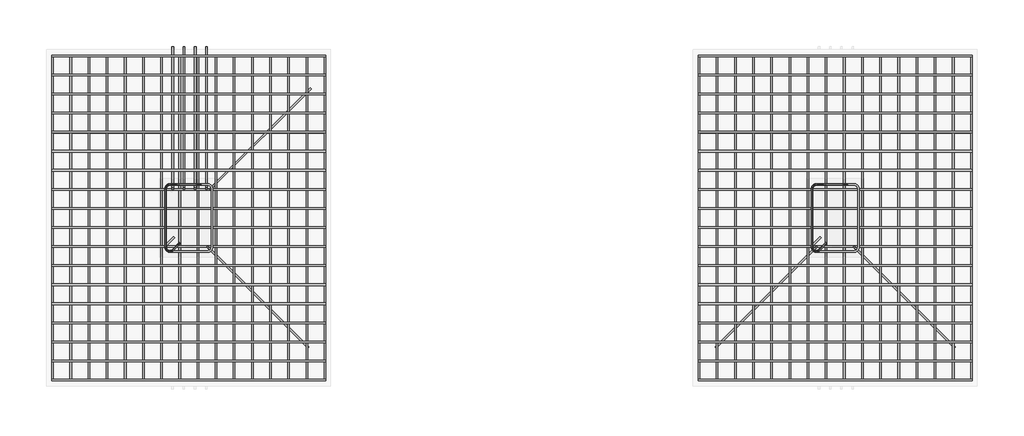
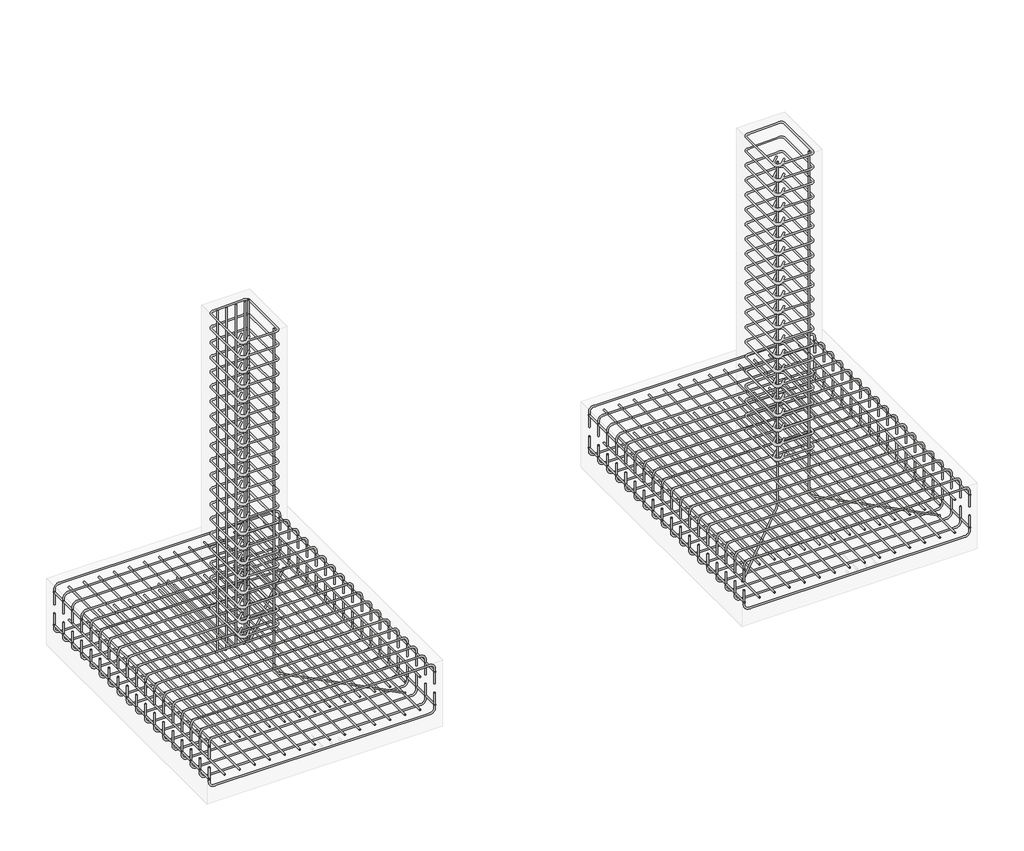
# One storey, part 10 of 33: 15 reinforcing bars.
"""IFC4 building model written with IfcOpenShell, lengths in millimetres."""

from ifc_helpers import new_model, si_unit, point, frame, origin, place, context, project, spatial, polyline, circle_curve, trimmed, segment, composite_curve, source, transform, mapped, element, save
from ifc_brep_helpers import swept_disk

model = new_model("IFC4")

# Units and contexts
model_context = context("Model", 3, world=origin())
ifc_project = project(units=[si_unit("LENGTHUNIT", "METRE", prefix="MILLI")], contexts=[model_context])

# Site, building, storey
site = spatial("IfcSite", under=ifc_project)
building = spatial("IfcBuilding", under=site)
storey = spatial("IfcBuildingStorey", under=building, Elevation=-3000.0)

# Reinforcing bars
placement = place(None, origin())
reinforcing_bar_shape = source(origin(), model_context, "Body", "SolidModel", [
    swept_disk(composite_curve([segment(polyline([(14306.5357258, -2044.0608134, -3240.0), (14306.5357258, -2044.0608134, -3092.7)]), True, "CONTINUOUS"), segment(trimmed(circle_curve(frame((14352.8857258, -2044.0608134, -3092.7), z_axis=(0.0, 1.0, 0.0), x_axis=(-46.350000000000364, 0.0, 0.0)), 46.35), [point((14306.5357258, -2044.0608134, -3092.7))], [point((14352.8857258, -2044.0608134, -3046.35))], True, "CARTESIAN"), True, "CONTINUOUS"), segment(polyline([(14352.8857258, -2044.0608134, -3046.35), (16367.4857258, -2044.0608134, -3046.35)]), True, "CONTINUOUS"), segment(trimmed(circle_curve(frame((16367.4857258, -2044.0608134, -3092.7), z_axis=(0.0, 1.0, 0.0), x_axis=(0.0, 0.0, 46.34999999999991)), 46.35), [point((16367.4857258, -2044.0608134, -3046.35))], [point((16413.8357258, -2044.0608134, -3092.7))], True, "CARTESIAN"), True, "CONTINUOUS"), segment(polyline([(16413.8357258, -2044.0608134, -3092.7), (16413.8357258, -2044.0608134, -3240.0)]), True, "CONTINUOUS")], self_intersect=False), 6.35),
])
element("IfcReinforcingBar", 1, at=placement, inside=storey, context=model_context, shape_type="MappedRepresentation", body=[
    mapped(reinforcing_bar_shape, transform((0.0, 0.0, 0.0), x_axis=(1.0, 0.0, 0.0), y_axis=(0.0, 1.0, 0.0), z_axis=(0.0, 0.0, 1.0))),
    mapped(reinforcing_bar_shape, transform((0.0, -147.4882353, 0.0), x_axis=(1.0, 0.0, 0.0), y_axis=(0.0, 1.0, 0.0), z_axis=(0.0, 0.0, 1.0))),
    mapped(reinforcing_bar_shape, transform((0.0, -294.9764706, 0.0), x_axis=(1.0, 0.0, 0.0), y_axis=(0.0, 1.0, 0.0), z_axis=(0.0, 0.0, 1.0))),
    mapped(reinforcing_bar_shape, transform((0.0, -442.4647059, 0.0), x_axis=(1.0, 0.0, 0.0), y_axis=(0.0, 1.0, 0.0), z_axis=(0.0, 0.0, 1.0))),
    mapped(reinforcing_bar_shape, transform((0.0, -589.9529412, 0.0), x_axis=(1.0, 0.0, 0.0), y_axis=(0.0, 1.0, 0.0), z_axis=(0.0, 0.0, 1.0))),
    mapped(reinforcing_bar_shape, transform((0.0, -737.4411765, 0.0), x_axis=(1.0, 0.0, 0.0), y_axis=(0.0, 1.0, 0.0), z_axis=(0.0, 0.0, 1.0))),
    mapped(reinforcing_bar_shape, transform((0.0, -884.9294118, 0.0), x_axis=(1.0, 0.0, 0.0), y_axis=(0.0, 1.0, 0.0), z_axis=(0.0, 0.0, 1.0))),
    mapped(reinforcing_bar_shape, transform((0.0, -1032.4176471, 0.0), x_axis=(1.0, 0.0, 0.0), y_axis=(0.0, 1.0, 0.0), z_axis=(0.0, 0.0, 1.0))),
    mapped(reinforcing_bar_shape, transform((0.0, -1179.9058824, 0.0), x_axis=(1.0, 0.0, 0.0), y_axis=(0.0, 1.0, 0.0), z_axis=(0.0, 0.0, 1.0))),
    mapped(reinforcing_bar_shape, transform((0.0, -1327.3941176, 0.0), x_axis=(1.0, 0.0, 0.0), y_axis=(0.0, 1.0, 0.0), z_axis=(0.0, 0.0, 1.0))),
    mapped(reinforcing_bar_shape, transform((0.0, -1474.8823529, 0.0), x_axis=(1.0, 0.0, 0.0), y_axis=(0.0, 1.0, 0.0), z_axis=(0.0, 0.0, 1.0))),
    mapped(reinforcing_bar_shape, transform((0.0, -1622.3705882, 0.0), x_axis=(1.0, 0.0, 0.0), y_axis=(0.0, 1.0, 0.0), z_axis=(0.0, 0.0, 1.0))),
    mapped(reinforcing_bar_shape, transform((0.0, -1769.8588235, 0.0), x_axis=(1.0, 0.0, 0.0), y_axis=(0.0, 1.0, 0.0), z_axis=(0.0, 0.0, 1.0))),
    mapped(reinforcing_bar_shape, transform((0.0, -1917.3470588, 0.0), x_axis=(1.0, 0.0, 0.0), y_axis=(0.0, 1.0, 0.0), z_axis=(0.0, 0.0, 1.0))),
    mapped(reinforcing_bar_shape, transform((0.0, -2064.8352941, 0.0), x_axis=(1.0, 0.0, 0.0), y_axis=(0.0, 1.0, 0.0), z_axis=(0.0, 0.0, 1.0))),
    mapped(reinforcing_bar_shape, transform((0.0, -2212.3235294, 0.0), x_axis=(1.0, 0.0, 0.0), y_axis=(0.0, 1.0, 0.0), z_axis=(0.0, 0.0, 1.0))),
    mapped(reinforcing_bar_shape, transform((0.0, -2359.8117647, 0.0), x_axis=(1.0, 0.0, 0.0), y_axis=(0.0, 1.0, 0.0), z_axis=(0.0, 0.0, 1.0))),
    mapped(reinforcing_bar_shape, transform((0.0, -2507.3, 0.0), x_axis=(1.0, 0.0, 0.0), y_axis=(0.0, 1.0, 0.0), z_axis=(0.0, 0.0, 1.0))),
])
reinforcing_bar_2_shape = source(origin(), model_context, "Body", "SolidModel", [
    swept_disk(composite_curve([segment(polyline([(16413.8357258, -2044.0608134, -3330.080452), (16413.8357258, -2044.0608134, -3477.380452)]), True, "CONTINUOUS"), segment(trimmed(circle_curve(frame((16367.4857258, -2044.0608134, -3477.380452), z_axis=(0.0, 1.0, 0.0), x_axis=(46.350000000000364, 0.0, 0.0)), 46.35), [point((16413.8357258, -2044.0608134, -3477.380452))], [point((16367.4857258, -2044.0608134, -3523.730452))], True, "CARTESIAN"), True, "CONTINUOUS"), segment(polyline([(16367.4857258, -2044.0608134, -3523.730452), (14352.8857258, -2044.0608134, -3523.730452)]), True, "CONTINUOUS"), segment(trimmed(circle_curve(frame((14352.8857258, -2044.0608134, -3477.380452), z_axis=(0.0, 1.0, 0.0), x_axis=(0.0, 0.0, -46.34999999999991)), 46.35), [point((14352.8857258, -2044.0608134, -3523.730452))], [point((14306.5357258, -2044.0608134, -3477.380452))], True, "CARTESIAN"), True, "CONTINUOUS"), segment(polyline([(14306.5357258, -2044.0608134, -3477.380452), (14306.5357258, -2044.0608134, -3330.080452)]), True, "CONTINUOUS")], self_intersect=False), 6.35),
])
element("IfcReinforcingBar", 2, at=placement, inside=storey, context=model_context, shape_type="MappedRepresentation", body=[
    mapped(reinforcing_bar_2_shape, transform((0.0, 0.0, 0.0), x_axis=(1.0, 0.0, 0.0), y_axis=(0.0, 1.0, 0.0), z_axis=(0.0, 0.0, 1.0))),
    mapped(reinforcing_bar_2_shape, transform((0.0, -147.4882353, 0.0), x_axis=(1.0, 0.0, 0.0), y_axis=(0.0, 1.0, 0.0), z_axis=(0.0, 0.0, 1.0))),
    mapped(reinforcing_bar_2_shape, transform((0.0, -294.9764706, 0.0), x_axis=(1.0, 0.0, 0.0), y_axis=(0.0, 1.0, 0.0), z_axis=(0.0, 0.0, 1.0))),
    mapped(reinforcing_bar_2_shape, transform((0.0, -442.4647059, 0.0), x_axis=(1.0, 0.0, 0.0), y_axis=(0.0, 1.0, 0.0), z_axis=(0.0, 0.0, 1.0))),
    mapped(reinforcing_bar_2_shape, transform((0.0, -589.9529412, 0.0), x_axis=(1.0, 0.0, 0.0), y_axis=(0.0, 1.0, 0.0), z_axis=(0.0, 0.0, 1.0))),
    mapped(reinforcing_bar_2_shape, transform((0.0, -737.4411765, 0.0), x_axis=(1.0, 0.0, 0.0), y_axis=(0.0, 1.0, 0.0), z_axis=(0.0, 0.0, 1.0))),
    mapped(reinforcing_bar_2_shape, transform((0.0, -884.9294118, 0.0), x_axis=(1.0, 0.0, 0.0), y_axis=(0.0, 1.0, 0.0), z_axis=(0.0, 0.0, 1.0))),
    mapped(reinforcing_bar_2_shape, transform((0.0, -1032.4176471, 0.0), x_axis=(1.0, 0.0, 0.0), y_axis=(0.0, 1.0, 0.0), z_axis=(0.0, 0.0, 1.0))),
    mapped(reinforcing_bar_2_shape, transform((0.0, -1179.9058824, 0.0), x_axis=(1.0, 0.0, 0.0), y_axis=(0.0, 1.0, 0.0), z_axis=(0.0, 0.0, 1.0))),
    mapped(reinforcing_bar_2_shape, transform((0.0, -1327.3941176, 0.0), x_axis=(1.0, 0.0, 0.0), y_axis=(0.0, 1.0, 0.0), z_axis=(0.0, 0.0, 1.0))),
    mapped(reinforcing_bar_2_shape, transform((0.0, -1474.8823529, 0.0), x_axis=(1.0, 0.0, 0.0), y_axis=(0.0, 1.0, 0.0), z_axis=(0.0, 0.0, 1.0))),
    mapped(reinforcing_bar_2_shape, transform((0.0, -1622.3705882, 0.0), x_axis=(1.0, 0.0, 0.0), y_axis=(0.0, 1.0, 0.0), z_axis=(0.0, 0.0, 1.0))),
    mapped(reinforcing_bar_2_shape, transform((0.0, -1769.8588235, 0.0), x_axis=(1.0, 0.0, 0.0), y_axis=(0.0, 1.0, 0.0), z_axis=(0.0, 0.0, 1.0))),
    mapped(reinforcing_bar_2_shape, transform((0.0, -1917.3470588, 0.0), x_axis=(1.0, 0.0, 0.0), y_axis=(0.0, 1.0, 0.0), z_axis=(0.0, 0.0, 1.0))),
    mapped(reinforcing_bar_2_shape, transform((0.0, -2064.8352941, 0.0), x_axis=(1.0, 0.0, 0.0), y_axis=(0.0, 1.0, 0.0), z_axis=(0.0, 0.0, 1.0))),
    mapped(reinforcing_bar_2_shape, transform((0.0, -2212.3235294, 0.0), x_axis=(1.0, 0.0, 0.0), y_axis=(0.0, 1.0, 0.0), z_axis=(0.0, 0.0, 1.0))),
    mapped(reinforcing_bar_2_shape, transform((0.0, -2359.8117647, 0.0), x_axis=(1.0, 0.0, 0.0), y_axis=(0.0, 1.0, 0.0), z_axis=(0.0, 0.0, 1.0))),
    mapped(reinforcing_bar_2_shape, transform((0.0, -2507.3, 0.0), x_axis=(1.0, 0.0, 0.0), y_axis=(0.0, 1.0, 0.0), z_axis=(0.0, 0.0, 1.0))),
])
reinforcing_bar_3_shape = source(origin(), model_context, "Body", "SolidModel", [
    swept_disk(composite_curve([segment(polyline([(16413.8357258, -4557.7108134, -3447.8614173), (16413.8357258, -2037.7108134, -3447.8614173)]), True, "CONTINUOUS")], self_intersect=False), 6.35),
])
element("IfcReinforcingBar", 3, at=placement, inside=storey, context=model_context, shape_type="MappedRepresentation", body=[
    mapped(reinforcing_bar_3_shape, transform((0.0, 0.0, 0.0), x_axis=(1.0, 0.0, 0.0), y_axis=(0.0, 1.0, 0.0), z_axis=(0.0, 0.0, 1.0))),
    mapped(reinforcing_bar_3_shape, transform((-140.4866667, 0.0, 0.0), x_axis=(1.0, 0.0, 0.0), y_axis=(0.0, 1.0, 0.0), z_axis=(0.0, 0.0, 1.0))),
    mapped(reinforcing_bar_3_shape, transform((-280.9733333, 0.0, 0.0), x_axis=(1.0, 0.0, 0.0), y_axis=(0.0, 1.0, 0.0), z_axis=(0.0, 0.0, 1.0))),
    mapped(reinforcing_bar_3_shape, transform((-421.46, 0.0, 0.0), x_axis=(1.0, 0.0, 0.0), y_axis=(0.0, 1.0, 0.0), z_axis=(0.0, 0.0, 1.0))),
    mapped(reinforcing_bar_3_shape, transform((-561.9466667, 0.0, 0.0), x_axis=(1.0, 0.0, 0.0), y_axis=(0.0, 1.0, 0.0), z_axis=(0.0, 0.0, 1.0))),
    mapped(reinforcing_bar_3_shape, transform((-702.4333333, 0.0, 0.0), x_axis=(1.0, 0.0, 0.0), y_axis=(0.0, 1.0, 0.0), z_axis=(0.0, 0.0, 1.0))),
    mapped(reinforcing_bar_3_shape, transform((-842.92, 0.0, 0.0), x_axis=(1.0, 0.0, 0.0), y_axis=(0.0, 1.0, 0.0), z_axis=(0.0, 0.0, 1.0))),
    mapped(reinforcing_bar_3_shape, transform((-983.4066667, 0.0, 0.0), x_axis=(1.0, 0.0, 0.0), y_axis=(0.0, 1.0, 0.0), z_axis=(0.0, 0.0, 1.0))),
    mapped(reinforcing_bar_3_shape, transform((-1123.8933333, 0.0, 0.0), x_axis=(1.0, 0.0, 0.0), y_axis=(0.0, 1.0, 0.0), z_axis=(0.0, 0.0, 1.0))),
    mapped(reinforcing_bar_3_shape, transform((-1264.38, 0.0, 0.0), x_axis=(1.0, 0.0, 0.0), y_axis=(0.0, 1.0, 0.0), z_axis=(0.0, 0.0, 1.0))),
    mapped(reinforcing_bar_3_shape, transform((-1404.8666667, 0.0, 0.0), x_axis=(1.0, 0.0, 0.0), y_axis=(0.0, 1.0, 0.0), z_axis=(0.0, 0.0, 1.0))),
    mapped(reinforcing_bar_3_shape, transform((-1545.3533333, 0.0, 0.0), x_axis=(1.0, 0.0, 0.0), y_axis=(0.0, 1.0, 0.0), z_axis=(0.0, 0.0, 1.0))),
    mapped(reinforcing_bar_3_shape, transform((-1685.84, 0.0, 0.0), x_axis=(1.0, 0.0, 0.0), y_axis=(0.0, 1.0, 0.0), z_axis=(0.0, 0.0, 1.0))),
    mapped(reinforcing_bar_3_shape, transform((-1826.3266667, 0.0, 0.0), x_axis=(1.0, 0.0, 0.0), y_axis=(0.0, 1.0, 0.0), z_axis=(0.0, 0.0, 1.0))),
    mapped(reinforcing_bar_3_shape, transform((-1966.8133333, 0.0, 0.0), x_axis=(1.0, 0.0, 0.0), y_axis=(0.0, 1.0, 0.0), z_axis=(0.0, 0.0, 1.0))),
    mapped(reinforcing_bar_3_shape, transform((-2107.3, 0.0, 0.0), x_axis=(1.0, 0.0, 0.0), y_axis=(0.0, 1.0, 0.0), z_axis=(0.0, 0.0, 1.0))),
])
reinforcing_bar_4_shape = source(origin(), model_context, "Body", "SolidModel", [
    swept_disk(composite_curve([segment(polyline([(14306.5357258, -4557.7108134, -3122.7084113), (14306.5357258, -2037.7108134, -3122.7084113)]), True, "CONTINUOUS")], self_intersect=False), 6.35),
])
element("IfcReinforcingBar", 4, at=placement, inside=storey, context=model_context, shape_type="MappedRepresentation", body=[
    mapped(reinforcing_bar_4_shape, transform((0.0, 0.0, 0.0), x_axis=(1.0, 0.0, 0.0), y_axis=(0.0, 1.0, 0.0), z_axis=(0.0, 0.0, 1.0))),
    mapped(reinforcing_bar_4_shape, transform((140.4866667, 0.0, 0.0), x_axis=(1.0, 0.0, 0.0), y_axis=(0.0, 1.0, 0.0), z_axis=(0.0, 0.0, 1.0))),
    mapped(reinforcing_bar_4_shape, transform((280.9733333, 0.0, 0.0), x_axis=(1.0, 0.0, 0.0), y_axis=(0.0, 1.0, 0.0), z_axis=(0.0, 0.0, 1.0))),
    mapped(reinforcing_bar_4_shape, transform((421.46, 0.0, 0.0), x_axis=(1.0, 0.0, 0.0), y_axis=(0.0, 1.0, 0.0), z_axis=(0.0, 0.0, 1.0))),
    mapped(reinforcing_bar_4_shape, transform((561.9466667, 0.0, 0.0), x_axis=(1.0, 0.0, 0.0), y_axis=(0.0, 1.0, 0.0), z_axis=(0.0, 0.0, 1.0))),
    mapped(reinforcing_bar_4_shape, transform((702.4333333, 0.0, 0.0), x_axis=(1.0, 0.0, 0.0), y_axis=(0.0, 1.0, 0.0), z_axis=(0.0, 0.0, 1.0))),
    mapped(reinforcing_bar_4_shape, transform((842.92, 0.0, 0.0), x_axis=(1.0, 0.0, 0.0), y_axis=(0.0, 1.0, 0.0), z_axis=(0.0, 0.0, 1.0))),
    mapped(reinforcing_bar_4_shape, transform((983.4066667, 0.0, 0.0), x_axis=(1.0, 0.0, 0.0), y_axis=(0.0, 1.0, 0.0), z_axis=(0.0, 0.0, 1.0))),
    mapped(reinforcing_bar_4_shape, transform((1123.8933333, 0.0, 0.0), x_axis=(1.0, 0.0, 0.0), y_axis=(0.0, 1.0, 0.0), z_axis=(0.0, 0.0, 1.0))),
    mapped(reinforcing_bar_4_shape, transform((1264.38, 0.0, 0.0), x_axis=(1.0, 0.0, 0.0), y_axis=(0.0, 1.0, 0.0), z_axis=(0.0, 0.0, 1.0))),
    mapped(reinforcing_bar_4_shape, transform((1404.8666667, 0.0, 0.0), x_axis=(1.0, 0.0, 0.0), y_axis=(0.0, 1.0, 0.0), z_axis=(0.0, 0.0, 1.0))),
    mapped(reinforcing_bar_4_shape, transform((1545.3533333, 0.0, 0.0), x_axis=(1.0, 0.0, 0.0), y_axis=(0.0, 1.0, 0.0), z_axis=(0.0, 0.0, 1.0))),
    mapped(reinforcing_bar_4_shape, transform((1685.84, 0.0, 0.0), x_axis=(1.0, 0.0, 0.0), y_axis=(0.0, 1.0, 0.0), z_axis=(0.0, 0.0, 1.0))),
    mapped(reinforcing_bar_4_shape, transform((1826.3266667, 0.0, 0.0), x_axis=(1.0, 0.0, 0.0), y_axis=(0.0, 1.0, 0.0), z_axis=(0.0, 0.0, 1.0))),
    mapped(reinforcing_bar_4_shape, transform((1966.8133333, 0.0, 0.0), x_axis=(1.0, 0.0, 0.0), y_axis=(0.0, 1.0, 0.0), z_axis=(0.0, 0.0, 1.0))),
    mapped(reinforcing_bar_4_shape, transform((2107.3, 0.0, 0.0), x_axis=(1.0, 0.0, 0.0), y_axis=(0.0, 1.0, 0.0), z_axis=(0.0, 0.0, 1.0))),
])
reinforcing_bar_5_shape = source(origin(), model_context, "Body", "SolidModel", [
    swept_disk(composite_curve([segment(polyline([(9306.5357258, -2044.0608134, -3240.0), (9306.5357258, -2044.0608134, -3092.7)]), True, "CONTINUOUS"), segment(trimmed(circle_curve(frame((9352.8857258, -2044.0608134, -3092.7), z_axis=(0.0, 1.0, 0.0), x_axis=(-46.350000000000364, 0.0, 0.0)), 46.35), [point((9306.5357258, -2044.0608134, -3092.7))], [point((9352.8857258, -2044.0608134, -3046.35))], True, "CARTESIAN"), True, "CONTINUOUS"), segment(polyline([(9352.8857258, -2044.0608134, -3046.35), (11367.4857258, -2044.0608134, -3046.35)]), True, "CONTINUOUS"), segment(trimmed(circle_curve(frame((11367.4857258, -2044.0608134, -3092.7), z_axis=(0.0, 1.0, 0.0), x_axis=(0.0, 0.0, 46.34999999999991)), 46.35), [point((11367.4857258, -2044.0608134, -3046.35))], [point((11413.8357258, -2044.0608134, -3092.7))], True, "CARTESIAN"), True, "CONTINUOUS"), segment(polyline([(11413.8357258, -2044.0608134, -3092.7), (11413.8357258, -2044.0608134, -3240.0)]), True, "CONTINUOUS")], self_intersect=False), 6.35),
])
element("IfcReinforcingBar", 5, at=placement, inside=storey, context=model_context, shape_type="MappedRepresentation", body=[
    mapped(reinforcing_bar_5_shape, transform((0.0, 0.0, 0.0), x_axis=(1.0, 0.0, 0.0), y_axis=(0.0, 1.0, 0.0), z_axis=(0.0, 0.0, 1.0))),
    mapped(reinforcing_bar_5_shape, transform((0.0, -147.4882353, 0.0), x_axis=(1.0, 0.0, 0.0), y_axis=(0.0, 1.0, 0.0), z_axis=(0.0, 0.0, 1.0))),
    mapped(reinforcing_bar_5_shape, transform((0.0, -294.9764706, 0.0), x_axis=(1.0, 0.0, 0.0), y_axis=(0.0, 1.0, 0.0), z_axis=(0.0, 0.0, 1.0))),
    mapped(reinforcing_bar_5_shape, transform((0.0, -442.4647059, 0.0), x_axis=(1.0, 0.0, 0.0), y_axis=(0.0, 1.0, 0.0), z_axis=(0.0, 0.0, 1.0))),
    mapped(reinforcing_bar_5_shape, transform((0.0, -589.9529412, 0.0), x_axis=(1.0, 0.0, 0.0), y_axis=(0.0, 1.0, 0.0), z_axis=(0.0, 0.0, 1.0))),
    mapped(reinforcing_bar_5_shape, transform((0.0, -737.4411765, 0.0), x_axis=(1.0, 0.0, 0.0), y_axis=(0.0, 1.0, 0.0), z_axis=(0.0, 0.0, 1.0))),
    mapped(reinforcing_bar_5_shape, transform((0.0, -884.9294118, 0.0), x_axis=(1.0, 0.0, 0.0), y_axis=(0.0, 1.0, 0.0), z_axis=(0.0, 0.0, 1.0))),
    mapped(reinforcing_bar_5_shape, transform((0.0, -1032.4176471, 0.0), x_axis=(1.0, 0.0, 0.0), y_axis=(0.0, 1.0, 0.0), z_axis=(0.0, 0.0, 1.0))),
    mapped(reinforcing_bar_5_shape, transform((0.0, -1179.9058824, 0.0), x_axis=(1.0, 0.0, 0.0), y_axis=(0.0, 1.0, 0.0), z_axis=(0.0, 0.0, 1.0))),
    mapped(reinforcing_bar_5_shape, transform((0.0, -1327.3941176, 0.0), x_axis=(1.0, 0.0, 0.0), y_axis=(0.0, 1.0, 0.0), z_axis=(0.0, 0.0, 1.0))),
    mapped(reinforcing_bar_5_shape, transform((0.0, -1474.8823529, 0.0), x_axis=(1.0, 0.0, 0.0), y_axis=(0.0, 1.0, 0.0), z_axis=(0.0, 0.0, 1.0))),
    mapped(reinforcing_bar_5_shape, transform((0.0, -1622.3705882, 0.0), x_axis=(1.0, 0.0, 0.0), y_axis=(0.0, 1.0, 0.0), z_axis=(0.0, 0.0, 1.0))),
    mapped(reinforcing_bar_5_shape, transform((0.0, -1769.8588235, 0.0), x_axis=(1.0, 0.0, 0.0), y_axis=(0.0, 1.0, 0.0), z_axis=(0.0, 0.0, 1.0))),
    mapped(reinforcing_bar_5_shape, transform((0.0, -1917.3470588, 0.0), x_axis=(1.0, 0.0, 0.0), y_axis=(0.0, 1.0, 0.0), z_axis=(0.0, 0.0, 1.0))),
    mapped(reinforcing_bar_5_shape, transform((0.0, -2064.8352941, 0.0), x_axis=(1.0, 0.0, 0.0), y_axis=(0.0, 1.0, 0.0), z_axis=(0.0, 0.0, 1.0))),
    mapped(reinforcing_bar_5_shape, transform((0.0, -2212.3235294, 0.0), x_axis=(1.0, 0.0, 0.0), y_axis=(0.0, 1.0, 0.0), z_axis=(0.0, 0.0, 1.0))),
    mapped(reinforcing_bar_5_shape, transform((0.0, -2359.8117647, 0.0), x_axis=(1.0, 0.0, 0.0), y_axis=(0.0, 1.0, 0.0), z_axis=(0.0, 0.0, 1.0))),
    mapped(reinforcing_bar_5_shape, transform((0.0, -2507.3, 0.0), x_axis=(1.0, 0.0, 0.0), y_axis=(0.0, 1.0, 0.0), z_axis=(0.0, 0.0, 1.0))),
])
reinforcing_bar_6_shape = source(origin(), model_context, "Body", "SolidModel", [
    swept_disk(composite_curve([segment(polyline([(11413.8357258, -2044.0608134, -3330.080452), (11413.8357258, -2044.0608134, -3477.380452)]), True, "CONTINUOUS"), segment(trimmed(circle_curve(frame((11367.4857258, -2044.0608134, -3477.380452), z_axis=(0.0, 1.0, 0.0), x_axis=(46.350000000000364, 0.0, 0.0)), 46.35), [point((11413.8357258, -2044.0608134, -3477.380452))], [point((11367.4857258, -2044.0608134, -3523.730452))], True, "CARTESIAN"), True, "CONTINUOUS"), segment(polyline([(11367.4857258, -2044.0608134, -3523.730452), (9352.8857258, -2044.0608134, -3523.730452)]), True, "CONTINUOUS"), segment(trimmed(circle_curve(frame((9352.8857258, -2044.0608134, -3477.380452), z_axis=(0.0, 1.0, 0.0), x_axis=(0.0, 0.0, -46.34999999999991)), 46.35), [point((9352.8857258, -2044.0608134, -3523.730452))], [point((9306.5357258, -2044.0608134, -3477.380452))], True, "CARTESIAN"), True, "CONTINUOUS"), segment(polyline([(9306.5357258, -2044.0608134, -3477.380452), (9306.5357258, -2044.0608134, -3330.080452)]), True, "CONTINUOUS")], self_intersect=False), 6.35),
])
element("IfcReinforcingBar", 6, at=placement, inside=storey, context=model_context, shape_type="MappedRepresentation", body=[
    mapped(reinforcing_bar_6_shape, transform((0.0, 0.0, 0.0), x_axis=(1.0, 0.0, 0.0), y_axis=(0.0, 1.0, 0.0), z_axis=(0.0, 0.0, 1.0))),
    mapped(reinforcing_bar_6_shape, transform((0.0, -147.4882353, 0.0), x_axis=(1.0, 0.0, 0.0), y_axis=(0.0, 1.0, 0.0), z_axis=(0.0, 0.0, 1.0))),
    mapped(reinforcing_bar_6_shape, transform((0.0, -294.9764706, 0.0), x_axis=(1.0, 0.0, 0.0), y_axis=(0.0, 1.0, 0.0), z_axis=(0.0, 0.0, 1.0))),
    mapped(reinforcing_bar_6_shape, transform((0.0, -442.4647059, 0.0), x_axis=(1.0, 0.0, 0.0), y_axis=(0.0, 1.0, 0.0), z_axis=(0.0, 0.0, 1.0))),
    mapped(reinforcing_bar_6_shape, transform((0.0, -589.9529412, 0.0), x_axis=(1.0, 0.0, 0.0), y_axis=(0.0, 1.0, 0.0), z_axis=(0.0, 0.0, 1.0))),
    mapped(reinforcing_bar_6_shape, transform((0.0, -737.4411765, 0.0), x_axis=(1.0, 0.0, 0.0), y_axis=(0.0, 1.0, 0.0), z_axis=(0.0, 0.0, 1.0))),
    mapped(reinforcing_bar_6_shape, transform((0.0, -884.9294118, 0.0), x_axis=(1.0, 0.0, 0.0), y_axis=(0.0, 1.0, 0.0), z_axis=(0.0, 0.0, 1.0))),
    mapped(reinforcing_bar_6_shape, transform((0.0, -1032.4176471, 0.0), x_axis=(1.0, 0.0, 0.0), y_axis=(0.0, 1.0, 0.0), z_axis=(0.0, 0.0, 1.0))),
    mapped(reinforcing_bar_6_shape, transform((0.0, -1179.9058824, 0.0), x_axis=(1.0, 0.0, 0.0), y_axis=(0.0, 1.0, 0.0), z_axis=(0.0, 0.0, 1.0))),
    mapped(reinforcing_bar_6_shape, transform((0.0, -1327.3941176, 0.0), x_axis=(1.0, 0.0, 0.0), y_axis=(0.0, 1.0, 0.0), z_axis=(0.0, 0.0, 1.0))),
    mapped(reinforcing_bar_6_shape, transform((0.0, -1474.8823529, 0.0), x_axis=(1.0, 0.0, 0.0), y_axis=(0.0, 1.0, 0.0), z_axis=(0.0, 0.0, 1.0))),
    mapped(reinforcing_bar_6_shape, transform((0.0, -1622.3705882, 0.0), x_axis=(1.0, 0.0, 0.0), y_axis=(0.0, 1.0, 0.0), z_axis=(0.0, 0.0, 1.0))),
    mapped(reinforcing_bar_6_shape, transform((0.0, -1769.8588235, 0.0), x_axis=(1.0, 0.0, 0.0), y_axis=(0.0, 1.0, 0.0), z_axis=(0.0, 0.0, 1.0))),
    mapped(reinforcing_bar_6_shape, transform((0.0, -1917.3470588, 0.0), x_axis=(1.0, 0.0, 0.0), y_axis=(0.0, 1.0, 0.0), z_axis=(0.0, 0.0, 1.0))),
    mapped(reinforcing_bar_6_shape, transform((0.0, -2064.8352941, 0.0), x_axis=(1.0, 0.0, 0.0), y_axis=(0.0, 1.0, 0.0), z_axis=(0.0, 0.0, 1.0))),
    mapped(reinforcing_bar_6_shape, transform((0.0, -2212.3235294, 0.0), x_axis=(1.0, 0.0, 0.0), y_axis=(0.0, 1.0, 0.0), z_axis=(0.0, 0.0, 1.0))),
    mapped(reinforcing_bar_6_shape, transform((0.0, -2359.8117647, 0.0), x_axis=(1.0, 0.0, 0.0), y_axis=(0.0, 1.0, 0.0), z_axis=(0.0, 0.0, 1.0))),
    mapped(reinforcing_bar_6_shape, transform((0.0, -2507.3, 0.0), x_axis=(1.0, 0.0, 0.0), y_axis=(0.0, 1.0, 0.0), z_axis=(0.0, 0.0, 1.0))),
])
reinforcing_bar_7_shape = source(origin(), model_context, "Body", "SolidModel", [
    swept_disk(composite_curve([segment(polyline([(11413.8357258, -4557.7108134, -3447.8614173), (11413.8357258, -2037.7108134, -3447.8614173)]), True, "CONTINUOUS")], self_intersect=False), 6.35),
])
element("IfcReinforcingBar", 7, at=placement, inside=storey, context=model_context, shape_type="MappedRepresentation", body=[
    mapped(reinforcing_bar_7_shape, transform((0.0, 0.0, 0.0), x_axis=(1.0, 0.0, 0.0), y_axis=(0.0, 1.0, 0.0), z_axis=(0.0, 0.0, 1.0))),
    mapped(reinforcing_bar_7_shape, transform((-140.4866667, 0.0, 0.0), x_axis=(1.0, 0.0, 0.0), y_axis=(0.0, 1.0, 0.0), z_axis=(0.0, 0.0, 1.0))),
    mapped(reinforcing_bar_7_shape, transform((-280.9733333, 0.0, 0.0), x_axis=(1.0, 0.0, 0.0), y_axis=(0.0, 1.0, 0.0), z_axis=(0.0, 0.0, 1.0))),
    mapped(reinforcing_bar_7_shape, transform((-421.46, 0.0, 0.0), x_axis=(1.0, 0.0, 0.0), y_axis=(0.0, 1.0, 0.0), z_axis=(0.0, 0.0, 1.0))),
    mapped(reinforcing_bar_7_shape, transform((-561.9466667, 0.0, 0.0), x_axis=(1.0, 0.0, 0.0), y_axis=(0.0, 1.0, 0.0), z_axis=(0.0, 0.0, 1.0))),
    mapped(reinforcing_bar_7_shape, transform((-702.4333333, 0.0, 0.0), x_axis=(1.0, 0.0, 0.0), y_axis=(0.0, 1.0, 0.0), z_axis=(0.0, 0.0, 1.0))),
    mapped(reinforcing_bar_7_shape, transform((-842.92, 0.0, 0.0), x_axis=(1.0, 0.0, 0.0), y_axis=(0.0, 1.0, 0.0), z_axis=(0.0, 0.0, 1.0))),
    mapped(reinforcing_bar_7_shape, transform((-983.4066667, 0.0, 0.0), x_axis=(1.0, 0.0, 0.0), y_axis=(0.0, 1.0, 0.0), z_axis=(0.0, 0.0, 1.0))),
    mapped(reinforcing_bar_7_shape, transform((-1123.8933333, 0.0, 0.0), x_axis=(1.0, 0.0, 0.0), y_axis=(0.0, 1.0, 0.0), z_axis=(0.0, 0.0, 1.0))),
    mapped(reinforcing_bar_7_shape, transform((-1264.38, 0.0, 0.0), x_axis=(1.0, 0.0, 0.0), y_axis=(0.0, 1.0, 0.0), z_axis=(0.0, 0.0, 1.0))),
    mapped(reinforcing_bar_7_shape, transform((-1404.8666667, 0.0, 0.0), x_axis=(1.0, 0.0, 0.0), y_axis=(0.0, 1.0, 0.0), z_axis=(0.0, 0.0, 1.0))),
    mapped(reinforcing_bar_7_shape, transform((-1545.3533333, 0.0, 0.0), x_axis=(1.0, 0.0, 0.0), y_axis=(0.0, 1.0, 0.0), z_axis=(0.0, 0.0, 1.0))),
    mapped(reinforcing_bar_7_shape, transform((-1685.84, 0.0, 0.0), x_axis=(1.0, 0.0, 0.0), y_axis=(0.0, 1.0, 0.0), z_axis=(0.0, 0.0, 1.0))),
    mapped(reinforcing_bar_7_shape, transform((-1826.3266667, 0.0, 0.0), x_axis=(1.0, 0.0, 0.0), y_axis=(0.0, 1.0, 0.0), z_axis=(0.0, 0.0, 1.0))),
    mapped(reinforcing_bar_7_shape, transform((-1966.8133333, 0.0, 0.0), x_axis=(1.0, 0.0, 0.0), y_axis=(0.0, 1.0, 0.0), z_axis=(0.0, 0.0, 1.0))),
    mapped(reinforcing_bar_7_shape, transform((-2107.3, 0.0, 0.0), x_axis=(1.0, 0.0, 0.0), y_axis=(0.0, 1.0, 0.0), z_axis=(0.0, 0.0, 1.0))),
])
reinforcing_bar_8_shape = source(origin(), model_context, "Body", "SolidModel", [
    swept_disk(composite_curve([segment(polyline([(9306.5357258, -4557.7108134, -3122.7084113), (9306.5357258, -2037.7108134, -3122.7084113)]), True, "CONTINUOUS")], self_intersect=False), 6.35),
])
element("IfcReinforcingBar", 8, at=placement, inside=storey, context=model_context, shape_type="MappedRepresentation", body=[
    mapped(reinforcing_bar_8_shape, transform((0.0, 0.0, 0.0), x_axis=(1.0, 0.0, 0.0), y_axis=(0.0, 1.0, 0.0), z_axis=(0.0, 0.0, 1.0))),
    mapped(reinforcing_bar_8_shape, transform((140.4866667, 0.0, 0.0), x_axis=(1.0, 0.0, 0.0), y_axis=(0.0, 1.0, 0.0), z_axis=(0.0, 0.0, 1.0))),
    mapped(reinforcing_bar_8_shape, transform((280.9733333, 0.0, 0.0), x_axis=(1.0, 0.0, 0.0), y_axis=(0.0, 1.0, 0.0), z_axis=(0.0, 0.0, 1.0))),
    mapped(reinforcing_bar_8_shape, transform((421.46, 0.0, 0.0), x_axis=(1.0, 0.0, 0.0), y_axis=(0.0, 1.0, 0.0), z_axis=(0.0, 0.0, 1.0))),
    mapped(reinforcing_bar_8_shape, transform((561.9466667, 0.0, 0.0), x_axis=(1.0, 0.0, 0.0), y_axis=(0.0, 1.0, 0.0), z_axis=(0.0, 0.0, 1.0))),
    mapped(reinforcing_bar_8_shape, transform((702.4333333, 0.0, 0.0), x_axis=(1.0, 0.0, 0.0), y_axis=(0.0, 1.0, 0.0), z_axis=(0.0, 0.0, 1.0))),
    mapped(reinforcing_bar_8_shape, transform((842.92, 0.0, 0.0), x_axis=(1.0, 0.0, 0.0), y_axis=(0.0, 1.0, 0.0), z_axis=(0.0, 0.0, 1.0))),
    mapped(reinforcing_bar_8_shape, transform((983.4066667, 0.0, 0.0), x_axis=(1.0, 0.0, 0.0), y_axis=(0.0, 1.0, 0.0), z_axis=(0.0, 0.0, 1.0))),
    mapped(reinforcing_bar_8_shape, transform((1123.8933333, 0.0, 0.0), x_axis=(1.0, 0.0, 0.0), y_axis=(0.0, 1.0, 0.0), z_axis=(0.0, 0.0, 1.0))),
    mapped(reinforcing_bar_8_shape, transform((1264.38, 0.0, 0.0), x_axis=(1.0, 0.0, 0.0), y_axis=(0.0, 1.0, 0.0), z_axis=(0.0, 0.0, 1.0))),
    mapped(reinforcing_bar_8_shape, transform((1404.8666667, 0.0, 0.0), x_axis=(1.0, 0.0, 0.0), y_axis=(0.0, 1.0, 0.0), z_axis=(0.0, 0.0, 1.0))),
    mapped(reinforcing_bar_8_shape, transform((1545.3533333, 0.0, 0.0), x_axis=(1.0, 0.0, 0.0), y_axis=(0.0, 1.0, 0.0), z_axis=(0.0, 0.0, 1.0))),
    mapped(reinforcing_bar_8_shape, transform((1685.84, 0.0, 0.0), x_axis=(1.0, 0.0, 0.0), y_axis=(0.0, 1.0, 0.0), z_axis=(0.0, 0.0, 1.0))),
    mapped(reinforcing_bar_8_shape, transform((1826.3266667, 0.0, 0.0), x_axis=(1.0, 0.0, 0.0), y_axis=(0.0, 1.0, 0.0), z_axis=(0.0, 0.0, 1.0))),
    mapped(reinforcing_bar_8_shape, transform((1966.8133333, 0.0, 0.0), x_axis=(1.0, 0.0, 0.0), y_axis=(0.0, 1.0, 0.0), z_axis=(0.0, 0.0, 1.0))),
    mapped(reinforcing_bar_8_shape, transform((2107.3, 0.0, 0.0), x_axis=(1.0, 0.0, 0.0), y_axis=(0.0, 1.0, 0.0), z_axis=(0.0, 0.0, 1.0))),
])
reinforcing_bar_9_shape = source(origin(), model_context, "Body", "SolidModel", [
    swept_disk(composite_curve([segment(polyline([(10246.4614911, -3446.8994528, -2953.65), (10190.7179282, -3502.6430158, -2953.65)]), True, "CONTINUOUS"), segment(trimmed(circle_curve(frame((10212.8857258, -3524.8108134, -2953.65), z_axis=(0.0, 0.0, 1.0), x_axis=(-22.167797600000995, 22.167797600000085, 0.0)), 31.35), [point((10190.7179282, -3502.6430158, -2953.65))], [point((10212.8857258, -3556.1608134, -2953.65))], True, "CARTESIAN"), True, "CONTINUOUS"), segment(polyline([(10212.8857258, -3556.1608134, -2953.65), (10507.4857258, -3556.1608134, -2953.65)]), True, "CONTINUOUS"), segment(trimmed(circle_curve(frame((10507.4857258, -3524.8108134, -2953.65), z_axis=(0.0, 0.0, 1.0), x_axis=(0.0, -31.34999999999991, 0.0)), 31.35), [point((10507.4857258, -3556.1608134, -2953.65))], [point((10538.8357258, -3524.8108134, -2953.65))], True, "CARTESIAN"), True, "CONTINUOUS"), segment(polyline([(10538.8357258, -3524.8108134, -2953.65), (10538.8357258, -3070.6108134, -2953.65)]), True, "CONTINUOUS"), segment(trimmed(circle_curve(frame((10507.5055109, -3070.6108134, -2954.7636125), z_axis=(-0.0355219283344822, 0.0, 0.9993688971583016), x_axis=(31.33021489999919, 0.0, 1.1136124999998174)), 31.35), [point((10538.8357258, -3070.6108134, -2953.65))], [point((10507.5055109, -3039.2608134, -2954.7636125))], True, "CARTESIAN"), True, "CONTINUOUS"), segment(polyline([(10507.5055109, -3039.2608134, -2954.7636125), (10212.8659407, -3039.2608134, -2965.2363875)]), True, "CONTINUOUS"), segment(trimmed(circle_curve(frame((10212.8659407, -3070.6108134, -2965.2363875), z_axis=(-0.0355219283344822, 0.0, 0.9993688971583016), x_axis=(0.0, 31.34999999999991, 0.0)), 31.35), [point((10212.8659407, -3039.2608134, -2965.2363875))], [point((10181.5357258, -3070.6108134, -2966.35))], True, "CARTESIAN"), True, "CONTINUOUS"), segment(polyline([(10181.5357258, -3070.6108134, -2966.35), (10181.5357258, -3524.8108134, -2966.35)]), True, "CONTINUOUS"), segment(trimmed(circle_curve(frame((10212.8857258, -3524.8108134, -2966.35), z_axis=(0.0, 0.0, 1.0), x_axis=(-31.350000000000364, 0.0, 0.0)), 31.35), [point((10181.5357258, -3524.8108134, -2966.35))], [point((10235.0535234, -3546.978611, -2966.35))], True, "CARTESIAN"), True, "CONTINUOUS"), segment(polyline([(10235.0535234, -3546.978611, -2966.35), (10290.7970863, -3491.235048, -2966.35)]), True, "CONTINUOUS")], self_intersect=False), 6.35),
])
element("IfcReinforcingBar", 9, at=placement, inside=storey, context=model_context, shape_type="MappedRepresentation", body=[
    mapped(reinforcing_bar_9_shape, transform((0.0, 0.0, 0.0), x_axis=(1.0, 0.0, 0.0), y_axis=(0.0, 1.0, 0.0), z_axis=(0.0, 0.0, 1.0))),
    mapped(reinforcing_bar_9_shape, transform((0.0, 0.0, 145.365), x_axis=(1.0, 0.0, 0.0), y_axis=(0.0, 1.0, 0.0), z_axis=(0.0, 0.0, 1.0))),
    mapped(reinforcing_bar_9_shape, transform((0.0, 0.0, 290.73), x_axis=(1.0, 0.0, 0.0), y_axis=(0.0, 1.0, 0.0), z_axis=(0.0, 0.0, 1.0))),
    mapped(reinforcing_bar_9_shape, transform((0.0, 0.0, 436.095), x_axis=(1.0, 0.0, 0.0), y_axis=(0.0, 1.0, 0.0), z_axis=(0.0, 0.0, 1.0))),
    mapped(reinforcing_bar_9_shape, transform((0.0, 0.0, 581.46), x_axis=(1.0, 0.0, 0.0), y_axis=(0.0, 1.0, 0.0), z_axis=(0.0, 0.0, 1.0))),
    mapped(reinforcing_bar_9_shape, transform((0.0, 0.0, 726.825), x_axis=(1.0, 0.0, 0.0), y_axis=(0.0, 1.0, 0.0), z_axis=(0.0, 0.0, 1.0))),
    mapped(reinforcing_bar_9_shape, transform((0.0, 0.0, 872.19), x_axis=(1.0, 0.0, 0.0), y_axis=(0.0, 1.0, 0.0), z_axis=(0.0, 0.0, 1.0))),
    mapped(reinforcing_bar_9_shape, transform((0.0, 0.0, 1017.555), x_axis=(1.0, 0.0, 0.0), y_axis=(0.0, 1.0, 0.0), z_axis=(0.0, 0.0, 1.0))),
    mapped(reinforcing_bar_9_shape, transform((0.0, 0.0, 1162.92), x_axis=(1.0, 0.0, 0.0), y_axis=(0.0, 1.0, 0.0), z_axis=(0.0, 0.0, 1.0))),
    mapped(reinforcing_bar_9_shape, transform((0.0, 0.0, 1308.285), x_axis=(1.0, 0.0, 0.0), y_axis=(0.0, 1.0, 0.0), z_axis=(0.0, 0.0, 1.0))),
    mapped(reinforcing_bar_9_shape, transform((0.0, 0.0, 1453.65), x_axis=(1.0, 0.0, 0.0), y_axis=(0.0, 1.0, 0.0), z_axis=(0.0, 0.0, 1.0))),
    mapped(reinforcing_bar_9_shape, transform((0.0, 0.0, 1599.015), x_axis=(1.0, 0.0, 0.0), y_axis=(0.0, 1.0, 0.0), z_axis=(0.0, 0.0, 1.0))),
    mapped(reinforcing_bar_9_shape, transform((0.0, 0.0, 1744.38), x_axis=(1.0, 0.0, 0.0), y_axis=(0.0, 1.0, 0.0), z_axis=(0.0, 0.0, 1.0))),
    mapped(reinforcing_bar_9_shape, transform((0.0, 0.0, 1889.745), x_axis=(1.0, 0.0, 0.0), y_axis=(0.0, 1.0, 0.0), z_axis=(0.0, 0.0, 1.0))),
    mapped(reinforcing_bar_9_shape, transform((0.0, 0.0, 2035.11), x_axis=(1.0, 0.0, 0.0), y_axis=(0.0, 1.0, 0.0), z_axis=(0.0, 0.0, 1.0))),
    mapped(reinforcing_bar_9_shape, transform((0.0, 0.0, 2180.475), x_axis=(1.0, 0.0, 0.0), y_axis=(0.0, 1.0, 0.0), z_axis=(0.0, 0.0, 1.0))),
    mapped(reinforcing_bar_9_shape, transform((0.0, 0.0, 2325.84), x_axis=(1.0, 0.0, 0.0), y_axis=(0.0, 1.0, 0.0), z_axis=(0.0, 0.0, 1.0))),
    mapped(reinforcing_bar_9_shape, transform((0.0, 0.0, 2471.205), x_axis=(1.0, 0.0, 0.0), y_axis=(0.0, 1.0, 0.0), z_axis=(0.0, 0.0, 1.0))),
    mapped(reinforcing_bar_9_shape, transform((0.0, 0.0, 2616.57), x_axis=(1.0, 0.0, 0.0), y_axis=(0.0, 1.0, 0.0), z_axis=(0.0, 0.0, 1.0))),
    mapped(reinforcing_bar_9_shape, transform((0.0, 0.0, 2761.935), x_axis=(1.0, 0.0, 0.0), y_axis=(0.0, 1.0, 0.0), z_axis=(0.0, 0.0, 1.0))),
    mapped(reinforcing_bar_9_shape, transform((0.0, 0.0, 2907.3), x_axis=(1.0, 0.0, 0.0), y_axis=(0.0, 1.0, 0.0), z_axis=(0.0, 0.0, 1.0))),
])
element("IfcReinforcingBar", 10, at=placement, inside=storey, context=model_context, shape_type="SolidModel", body=[
    swept_disk(composite_curve([segment(polyline([(10507.1671301, -3521.6339414, -40.0), (10507.1671301, -3521.6339414, -3393.65)]), True, "CONTINUOUS"), segment(trimmed(circle_curve(frame((10539.9415294, -3554.4083407, -3393.65), z_axis=(-0.7071067811865493, -0.7071067811865459, 0.0), x_axis=(-32.77439929999855, 32.774399299999914, 0.0)), 46.35), [point((10507.1671301, -3521.6339414, -3393.65))], [point((10539.9415294, -3554.4083407, -3440.0))], True, "CARTESIAN"), True, "CONTINUOUS"), segment(polyline([(10539.9415294, -3554.4083407, -3440.0), (11284.9845894, -4299.4514007, -3440.0)]), True, "CONTINUOUS")], self_intersect=False), 6.35),
])
element("IfcReinforcingBar", 11, at=placement, inside=storey, context=model_context, shape_type="SolidModel", body=[
    swept_disk(composite_curve([segment(polyline([(10525.7684217, -3073.7876853, -30.2564663), (10525.7684217, -3073.7876853, -3383.9064663)]), True, "CONTINUOUS"), segment(trimmed(circle_curve(frame((10558.542821, -3041.013286, -3383.9064663), z_axis=(0.7071067811865493, -0.7071067811865459, 0.0), x_axis=(-32.77439929999855, -32.774399299999914, 0.0)), 46.35), [point((10525.7684217, -3073.7876853, -3383.9064663))], [point((10558.542821, -3041.013286, -3430.2564663))], True, "CARTESIAN"), True, "CONTINUOUS"), segment(polyline([(10558.542821, -3041.013286, -3430.2564663), (11303.585881, -2295.970226, -3430.2564663)]), True, "CONTINUOUS")], self_intersect=False), 6.35),
])
reinforcing_bar_10_shape = source(origin(), model_context, "Body", "SolidModel", [
    swept_disk(composite_curve([segment(polyline([(10236.1158322, -3071.9278134, -40.0), (10236.1158322, -3071.9278134, -3393.65)]), True, "CONTINUOUS"), segment(trimmed(circle_curve(frame((10236.1158322, -3025.5778134, -3393.65), z_axis=(1.0, 0.0, 0.0), x_axis=(0.0, -46.34999999999991, 0.0)), 46.35), [point((10236.1158322, -3071.9278134, -3393.65))], [point((10236.1158322, -3025.5778134, -3440.0))], True, "CARTESIAN"), True, "CONTINUOUS"), segment(polyline([(10236.1158322, -3025.5778134, -3440.0), (10236.1158322, -1971.9278134, -3440.0)]), True, "CONTINUOUS")], self_intersect=False), 6.35),
])
element("IfcReinforcingBar", 12, at=placement, inside=storey, context=model_context, shape_type="MappedRepresentation", body=[
    mapped(reinforcing_bar_10_shape, transform((0.0, 0.0, 0.0), x_axis=(1.0, 0.0, 0.0), y_axis=(0.0, 1.0, 0.0), z_axis=(0.0, 0.0, 1.0))),
    mapped(reinforcing_bar_10_shape, transform((86.8979716, 0.0, 0.0), x_axis=(1.0, 0.0, 0.0), y_axis=(0.0, 1.0, 0.0), z_axis=(0.0, 0.0, 1.0))),
    mapped(reinforcing_bar_10_shape, transform((173.7959432, 0.0, 0.0), x_axis=(1.0, 0.0, 0.0), y_axis=(0.0, 1.0, 0.0), z_axis=(0.0, 0.0, 1.0))),
    mapped(reinforcing_bar_10_shape, transform((260.6939148, 0.0, 0.0), x_axis=(1.0, 0.0, 0.0), y_axis=(0.0, 1.0, 0.0), z_axis=(0.0, 0.0, 1.0))),
])
reinforcing_bar_11_shape = source(origin(), model_context, "Body", "SolidModel", [
    swept_disk(composite_curve([segment(polyline([(15246.4614911, -3446.8994528, -2953.65), (15190.7179282, -3502.6430158, -2953.65)]), True, "CONTINUOUS"), segment(trimmed(circle_curve(frame((15212.8857258, -3524.8108134, -2953.65), z_axis=(0.0, 0.0, 1.0), x_axis=(-22.167797600000995, 22.167797600000085, 0.0)), 31.35), [point((15190.7179282, -3502.6430158, -2953.65))], [point((15212.8857258, -3556.1608134, -2953.65))], True, "CARTESIAN"), True, "CONTINUOUS"), segment(polyline([(15212.8857258, -3556.1608134, -2953.65), (15507.4857258, -3556.1608134, -2953.65)]), True, "CONTINUOUS"), segment(trimmed(circle_curve(frame((15507.4857258, -3524.8108134, -2953.65), z_axis=(0.0, 0.0, 1.0), x_axis=(0.0, -31.34999999999991, 0.0)), 31.35), [point((15507.4857258, -3556.1608134, -2953.65))], [point((15538.8357258, -3524.8108134, -2953.65))], True, "CARTESIAN"), True, "CONTINUOUS"), segment(polyline([(15538.8357258, -3524.8108134, -2953.65), (15538.8357258, -3070.6108134, -2953.65)]), True, "CONTINUOUS"), segment(trimmed(circle_curve(frame((15507.5055109, -3070.6108134, -2954.7636125), z_axis=(-0.0355219283344822, 0.0, 0.9993688971583016), x_axis=(31.33021489999919, 0.0, 1.1136124999998174)), 31.35), [point((15538.8357258, -3070.6108134, -2953.65))], [point((15507.5055109, -3039.2608134, -2954.7636125))], True, "CARTESIAN"), True, "CONTINUOUS"), segment(polyline([(15507.5055109, -3039.2608134, -2954.7636125), (15212.8659407, -3039.2608134, -2965.2363875)]), True, "CONTINUOUS"), segment(trimmed(circle_curve(frame((15212.8659407, -3070.6108134, -2965.2363875), z_axis=(-0.0355219283344822, 0.0, 0.9993688971583016), x_axis=(0.0, 31.34999999999991, 0.0)), 31.35), [point((15212.8659407, -3039.2608134, -2965.2363875))], [point((15181.5357258, -3070.6108134, -2966.35))], True, "CARTESIAN"), True, "CONTINUOUS"), segment(polyline([(15181.5357258, -3070.6108134, -2966.35), (15181.5357258, -3524.8108134, -2966.35)]), True, "CONTINUOUS"), segment(trimmed(circle_curve(frame((15212.8857258, -3524.8108134, -2966.35), z_axis=(0.0, 0.0, 1.0), x_axis=(-31.350000000000364, 0.0, 0.0)), 31.35), [point((15181.5357258, -3524.8108134, -2966.35))], [point((15235.0535234, -3546.978611, -2966.35))], True, "CARTESIAN"), True, "CONTINUOUS"), segment(polyline([(15235.0535234, -3546.978611, -2966.35), (15290.7970863, -3491.235048, -2966.35)]), True, "CONTINUOUS")], self_intersect=False), 6.35),
])
element("IfcReinforcingBar", 13, at=placement, inside=storey, context=model_context, shape_type="MappedRepresentation", body=[
    mapped(reinforcing_bar_11_shape, transform((0.0, 0.0, 0.0), x_axis=(1.0, 0.0, 0.0), y_axis=(0.0, 1.0, 0.0), z_axis=(0.0, 0.0, 1.0))),
    mapped(reinforcing_bar_11_shape, transform((0.0, 0.0, 145.365), x_axis=(1.0, 0.0, 0.0), y_axis=(0.0, 1.0, 0.0), z_axis=(0.0, 0.0, 1.0))),
    mapped(reinforcing_bar_11_shape, transform((0.0, 0.0, 290.73), x_axis=(1.0, 0.0, 0.0), y_axis=(0.0, 1.0, 0.0), z_axis=(0.0, 0.0, 1.0))),
    mapped(reinforcing_bar_11_shape, transform((0.0, 0.0, 436.095), x_axis=(1.0, 0.0, 0.0), y_axis=(0.0, 1.0, 0.0), z_axis=(0.0, 0.0, 1.0))),
    mapped(reinforcing_bar_11_shape, transform((0.0, 0.0, 581.46), x_axis=(1.0, 0.0, 0.0), y_axis=(0.0, 1.0, 0.0), z_axis=(0.0, 0.0, 1.0))),
    mapped(reinforcing_bar_11_shape, transform((0.0, 0.0, 726.825), x_axis=(1.0, 0.0, 0.0), y_axis=(0.0, 1.0, 0.0), z_axis=(0.0, 0.0, 1.0))),
    mapped(reinforcing_bar_11_shape, transform((0.0, 0.0, 872.19), x_axis=(1.0, 0.0, 0.0), y_axis=(0.0, 1.0, 0.0), z_axis=(0.0, 0.0, 1.0))),
    mapped(reinforcing_bar_11_shape, transform((0.0, 0.0, 1017.555), x_axis=(1.0, 0.0, 0.0), y_axis=(0.0, 1.0, 0.0), z_axis=(0.0, 0.0, 1.0))),
    mapped(reinforcing_bar_11_shape, transform((0.0, 0.0, 1162.92), x_axis=(1.0, 0.0, 0.0), y_axis=(0.0, 1.0, 0.0), z_axis=(0.0, 0.0, 1.0))),
    mapped(reinforcing_bar_11_shape, transform((0.0, 0.0, 1308.285), x_axis=(1.0, 0.0, 0.0), y_axis=(0.0, 1.0, 0.0), z_axis=(0.0, 0.0, 1.0))),
    mapped(reinforcing_bar_11_shape, transform((0.0, 0.0, 1453.65), x_axis=(1.0, 0.0, 0.0), y_axis=(0.0, 1.0, 0.0), z_axis=(0.0, 0.0, 1.0))),
    mapped(reinforcing_bar_11_shape, transform((0.0, 0.0, 1599.015), x_axis=(1.0, 0.0, 0.0), y_axis=(0.0, 1.0, 0.0), z_axis=(0.0, 0.0, 1.0))),
    mapped(reinforcing_bar_11_shape, transform((0.0, 0.0, 1744.38), x_axis=(1.0, 0.0, 0.0), y_axis=(0.0, 1.0, 0.0), z_axis=(0.0, 0.0, 1.0))),
    mapped(reinforcing_bar_11_shape, transform((0.0, 0.0, 1889.745), x_axis=(1.0, 0.0, 0.0), y_axis=(0.0, 1.0, 0.0), z_axis=(0.0, 0.0, 1.0))),
    mapped(reinforcing_bar_11_shape, transform((0.0, 0.0, 2035.11), x_axis=(1.0, 0.0, 0.0), y_axis=(0.0, 1.0, 0.0), z_axis=(0.0, 0.0, 1.0))),
    mapped(reinforcing_bar_11_shape, transform((0.0, 0.0, 2180.475), x_axis=(1.0, 0.0, 0.0), y_axis=(0.0, 1.0, 0.0), z_axis=(0.0, 0.0, 1.0))),
    mapped(reinforcing_bar_11_shape, transform((0.0, 0.0, 2325.84), x_axis=(1.0, 0.0, 0.0), y_axis=(0.0, 1.0, 0.0), z_axis=(0.0, 0.0, 1.0))),
    mapped(reinforcing_bar_11_shape, transform((0.0, 0.0, 2471.205), x_axis=(1.0, 0.0, 0.0), y_axis=(0.0, 1.0, 0.0), z_axis=(0.0, 0.0, 1.0))),
    mapped(reinforcing_bar_11_shape, transform((0.0, 0.0, 2616.57), x_axis=(1.0, 0.0, 0.0), y_axis=(0.0, 1.0, 0.0), z_axis=(0.0, 0.0, 1.0))),
    mapped(reinforcing_bar_11_shape, transform((0.0, 0.0, 2761.935), x_axis=(1.0, 0.0, 0.0), y_axis=(0.0, 1.0, 0.0), z_axis=(0.0, 0.0, 1.0))),
    mapped(reinforcing_bar_11_shape, transform((0.0, 0.0, 2907.3), x_axis=(1.0, 0.0, 0.0), y_axis=(0.0, 1.0, 0.0), z_axis=(0.0, 0.0, 1.0))),
])
element("IfcReinforcingBar", 14, at=placement, inside=storey, context=model_context, shape_type="SolidModel", body=[
    swept_disk(composite_curve([segment(polyline([(15213.2043214, -3521.6339414, -40.0), (15213.2043214, -3521.6339414, -3393.65)]), True, "CONTINUOUS"), segment(trimmed(circle_curve(frame((15180.4299221, -3554.4083407, -3393.65), z_axis=(-0.7071067811865446, 0.7071067811865505, 0.0), x_axis=(32.77439930000037, 32.774399299999914, 0.0)), 46.35), [point((15213.2043214, -3521.6339414, -3393.65))], [point((15180.4299221, -3554.4083407, -3440.0))], True, "CARTESIAN"), True, "CONTINUOUS"), segment(polyline([(15180.4299221, -3554.4083407, -3440.0), (14435.3868621, -4299.4514007, -3440.0)]), True, "CONTINUOUS")], self_intersect=False), 6.35),
])
element("IfcReinforcingBar", 15, at=placement, inside=storey, context=model_context, shape_type="SolidModel", body=[
    swept_disk(composite_curve([segment(polyline([(15507.1671301, -3521.6339414, -40.0), (15507.1671301, -3521.6339414, -3393.65)]), True, "CONTINUOUS"), segment(trimmed(circle_curve(frame((15539.9415294, -3554.4083407, -3393.65), z_axis=(-0.7071067811865493, -0.7071067811865459, 0.0), x_axis=(-32.77439929999855, 32.774399299999914, 0.0)), 46.35), [point((15507.1671301, -3521.6339414, -3393.65))], [point((15539.9415294, -3554.4083407, -3440.0))], True, "CARTESIAN"), True, "CONTINUOUS"), segment(polyline([(15539.9415294, -3554.4083407, -3440.0), (16284.9845894, -4299.4514007, -3440.0)]), True, "CONTINUOUS")], self_intersect=False), 6.35),
])

save(model, "model.ifc")

# Revit data of these elements
# Elements 1, 2, 3, 4, 5, 6, 7, 8, 9, 10, 11, 12, 13, 14, 15 (IfcReinforcingBar)
#   Phase Created = New Construction
